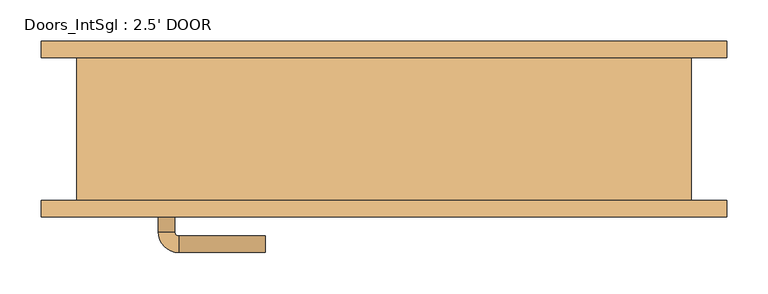
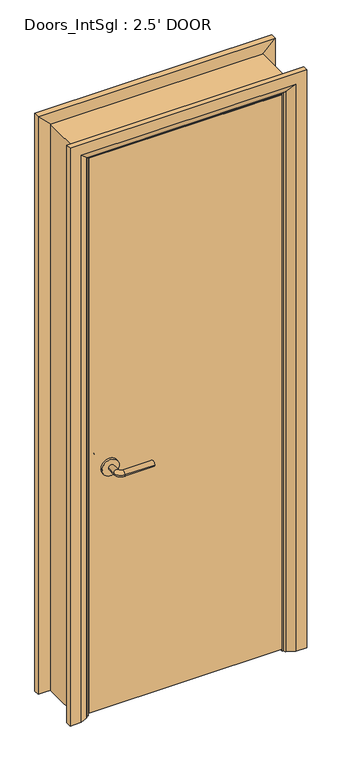
"""IFC4 building model written with IfcOpenShell, lengths in millimetres: door geometry, Doors_IntSgl : 2.5' DOOR."""

from ifc_helpers import new_model, si_unit, point, frame, frame_2d, origin, place, context, project, spatial, polyline, circle_curve, ellipse_curve, trimmed, segment, composite_curve, outline, extrude, faceted_brep, source, transform, mapped, element, save
from ifc_brep_helpers import plane_surface, cylinder_surface, revolved_surface, advanced_brep


def doors_intsgl_2_5_door_fd097d29(model_context):
    return source(origin(), model_context, "Body", "SolidModel", [
        advanced_brep(
        [(-274.0, -40.868, 900.0), (-254.0, -40.868, 900.0), (-274.0, -10.868, 900.0), (-254.0, -10.868, 900.0), (-249.0, -5.868, 900.0), (-249.0, 14.132, 900.0), (-144.0, 14.132, 900.0), (-144.0, -5.868, 900.0)],
        [
            (0, 1, circle_curve(frame((-264.0, -40.868, 900.0), z_axis=(0.0, -1.0, 0.0), x_axis=(1.0, 0.0, 0.0)), 10.0)),
            (1, 0, circle_curve(frame((-264.0, -40.868, 900.0), z_axis=(0.0, -1.0, 0.0), x_axis=(1.0, 0.0, 0.0)), 10.0)),
            (0, 2),
            (2, 3, circle_curve(frame((-264.0, -10.868, 900.0), z_axis=(0.0, -1.0, 0.0), x_axis=(1.0, 0.0, 0.0)), 10.0)),
            (3, 1),
            (3, 2, circle_curve(frame((-264.0, -10.868, 900.0), z_axis=(0.0, -1.0, 0.0), x_axis=(1.0, 0.0, 0.0)), 10.0)),
            (4, 3, circle_curve(frame((-249.0, -10.868, 900.0), z_axis=(0.0, 0.0, 1.0), x_axis=(-1.0, 0.0, 0.0)), 5.0)),
            (2, 5, circle_curve(frame((-249.0, -10.868, 900.0), z_axis=(0.0, 0.0, -1.0), x_axis=(-1.0, 0.0, 0.0)), 25.0)),
            (5, 4, circle_curve(frame((-249.0, 4.132, 900.0), z_axis=(-1.0, 0.0, 0.0), x_axis=(0.0, -1.0, 0.0)), 10.0)),
            (4, 5, circle_curve(frame((-249.0, 4.132, 900.0), z_axis=(-1.0, 0.0, 0.0), x_axis=(0.0, -1.0, 0.0)), 10.0)),
            (6, 7, circle_curve(frame((-144.0, 4.132, 900.0), z_axis=(1.0, 0.0, 0.0), x_axis=(0.0, -1.0, 0.0)), 10.0)),
            (7, 6, circle_curve(frame((-144.0, 4.132, 900.0), z_axis=(1.0, 0.0, 0.0), x_axis=(0.0, -1.0, 0.0)), 10.0)),
            (5, 6),
            (7, 4),
        ],
        [
            plane_surface(frame((-264.0, -40.868, 900.0), z_axis=(0.0, -1.0, 0.0), x_axis=(0.0, 0.0, 1.0))),
            cylinder_surface(frame((-264.0, -40.868, 900.0), z_axis=(0.0, -1.0, 0.0), x_axis=(1.0, 0.0, 0.0)), 10.0),
            revolved_surface(trimmed(ellipse_curve(frame((-264.0, -10.868, 900.0), z_axis=(0.0, -1.0, 0.0), x_axis=(1.0, 0.0, 0.0)), 10.0, 10.0), [point((-274.0, -10.868, 900.0))], [point((-254.0, -10.868, 900.0))], True, "CARTESIAN"), (-249.0, -10.868, 900.0), (0.0, 0.0, -1.0)),
            revolved_surface(trimmed(ellipse_curve(frame((-264.0, -10.868, 900.0), z_axis=(0.0, -1.0, 0.0), x_axis=(1.0, 0.0, 0.0)), 10.0, 10.0), [point((-254.0, -10.868, 900.0))], [point((-274.0, -10.868, 900.0))], True, "CARTESIAN"), (-249.0, -10.868, 900.0), (0.0, 0.0, -1.0)),
            plane_surface(frame((-144.0, 4.132, 900.0), z_axis=(1.0, 0.0, 0.0), x_axis=(0.0, 0.0, 1.0))),
            cylinder_surface(frame((-249.0, 4.132, 900.0), z_axis=(-1.0, 0.0, 0.0), x_axis=(0.0, -1.0, 0.0)), 10.0),
        ],
        [
            (0, [[1, 2]]),
            (1, [[-1, 3, 4, 5]]),
            (1, [[-2, -5, 6, -3]]),
            (2, [[7, -4, 8, 9]]),
            (3, [[-8, -6, -7, 10]]),
            (4, [[11, 12]]),
            (5, [[-9, 13, -12, 14]]),
            (5, [[-10, -14, -11, -13]]),
        ],
    ),
        extrude(outline(composite_curve([segment(trimmed(circle_curve(frame_2d((900.0, -266.5)), 30.0), [point((900.0, -296.5))], [point((900.0, -236.5))], False, "CARTESIAN"), True, "CONTINUOUS"), segment(trimmed(circle_curve(frame_2d((900.0, -266.5)), 30.0), [point((900.0, -236.5))], [point((900.0, -296.5))], False, "CARTESIAN"), True, "CONTINUOUS")], self_intersect=False)), frame((0.0, -48.868, 0.0), z_axis=(0.0, 1.0, 0.0), x_axis=(0.0, 0.0, 1.0)), (0.0, 0.0, 1.0), 8.0),
        advanced_brep(
        [(-274.0, -94.868, 900.0), (-254.0, -94.868, 900.0), (-254.0, -124.868, 900.0), (-274.0, -124.868, 900.0), (-249.0, -129.868, 900.0), (-249.0, -149.868, 900.0), (-144.0, -149.868, 900.0), (-144.0, -129.868, 900.0)],
        [
            (0, 1, circle_curve(frame((-264.0, -94.868, 900.0), z_axis=(0.0, 1.0, 0.0), x_axis=(1.0, 0.0, 0.0)), 10.0)),
            (1, 0, circle_curve(frame((-264.0, -94.868, 900.0), z_axis=(0.0, 1.0, 0.0), x_axis=(1.0, 0.0, 0.0)), 10.0)),
            (1, 2),
            (2, 3, circle_curve(frame((-264.0, -124.868, 900.0), z_axis=(0.0, 1.0, 0.0), x_axis=(1.0, 0.0, 0.0)), 10.0)),
            (3, 0),
            (3, 2, circle_curve(frame((-264.0, -124.868, 900.0), z_axis=(0.0, 1.0, 0.0), x_axis=(1.0, 0.0, 0.0)), 10.0)),
            (4, 5, circle_curve(frame((-249.0, -139.868, 900.0), z_axis=(-1.0, 0.0, 0.0), x_axis=(0.0, 1.0, 0.0)), 10.0)),
            (5, 3, circle_curve(frame((-249.0, -124.868, 900.0), z_axis=(0.0, 0.0, -1.0), x_axis=(-1.0, 0.0, 0.0)), 25.0)),
            (2, 4, circle_curve(frame((-249.0, -124.868, 900.0), z_axis=(0.0, 0.0, 1.0), x_axis=(-1.0, 0.0, 0.0)), 5.0)),
            (5, 4, circle_curve(frame((-249.0, -139.868, 900.0), z_axis=(-1.0, 0.0, 0.0), x_axis=(0.0, 1.0, 0.0)), 10.0)),
            (6, 7, circle_curve(frame((-144.0, -139.868, 900.0), z_axis=(1.0, 0.0, 0.0), x_axis=(0.0, 1.0, 0.0)), 10.0)),
            (7, 6, circle_curve(frame((-144.0, -139.868, 900.0), z_axis=(1.0, 0.0, 0.0), x_axis=(0.0, 1.0, 0.0)), 10.0)),
            (4, 7),
            (6, 5),
        ],
        [
            plane_surface(frame((-264.0, -94.868, 900.0), z_axis=(0.0, 1.0, 0.0), x_axis=(0.0, 0.0, 1.0))),
            cylinder_surface(frame((-264.0, -94.868, 900.0), z_axis=(0.0, 1.0, 0.0), x_axis=(1.0, 0.0, 0.0)), 10.0),
            revolved_surface(trimmed(ellipse_curve(frame((-264.0, -124.868, 900.0), z_axis=(0.0, -1.0, 0.0), x_axis=(1.0, 0.0, 0.0)), 10.0, 10.0), [point((-274.0, -124.868, 900.0))], [point((-254.0, -124.868, 900.0))], True, "CARTESIAN"), (-249.0, -124.868, 900.0), (0.0, 0.0, -1.0)),
            revolved_surface(trimmed(ellipse_curve(frame((-264.0, -124.868, 900.0), z_axis=(0.0, -1.0, 0.0), x_axis=(1.0, 0.0, 0.0)), 10.0, 10.0), [point((-254.0, -124.868, 900.0))], [point((-274.0, -124.868, 900.0))], True, "CARTESIAN"), (-249.0, -124.868, 900.0), (0.0, 0.0, -1.0)),
            plane_surface(frame((-144.0, -139.868, 900.0), z_axis=(1.0, 0.0, 0.0), x_axis=(0.0, 0.0, 1.0))),
            cylinder_surface(frame((-249.0, -139.868, 900.0), z_axis=(-1.0, 0.0, 0.0), x_axis=(0.0, 1.0, 0.0)), 10.0),
        ],
        [
            (0, [[1, 2]]),
            (1, [[3, 4, 5, -2]]),
            (1, [[-5, 6, -3, -1]]),
            (2, [[7, 8, -4, 9]]),
            (3, [[10, -9, -6, -8]]),
            (4, [[11, 12]]),
            (5, [[13, -11, 14, -7]]),
            (5, [[-14, -12, -13, -10]]),
        ],
    ),
        extrude(outline(composite_curve([segment(trimmed(circle_curve(frame_2d((900.0, -266.5)), 30.0), [point((900.0, -296.5))], [point((900.0, -236.5))], False, "CARTESIAN"), True, "CONTINUOUS"), segment(trimmed(circle_curve(frame_2d((900.0, -266.5)), 30.0), [point((900.0, -236.5))], [point((900.0, -296.5))], False, "CARTESIAN"), True, "CONTINUOUS")], self_intersect=False)), frame((0.0, -94.868, 0.0), z_axis=(0.0, 1.0, 0.0), x_axis=(0.0, 0.0, 1.0)), (0.0, 0.0, 1.0), 8.0),
        extrude(outline(polyline([(339.0, -48.868), (339.0, -86.868), (-339.0, -86.868), (-339.0, -48.868), (339.0, -48.868)])), frame((0.0, 0.0, 8.0), z_axis=(0.0, 0.0, 1.0), x_axis=(1.0, 0.0, 0.0)), (0.0, 0.0, 1.0), 2060.0),
        advanced_brep(
        [(416.0, -106.868, 0.0), (376.0, -106.868, 0.0), (350.0, -92.868, 0.0), (346.0, -86.868, 0.0), (416.0, -86.868, 0.0), (416.0, -86.868, 2145.0), (416.0, -106.868, 2145.0), (346.0, -86.868, 2075.0), (-346.0, -86.868, 2075.0), (-346.0, -86.868, 0.0), (-416.0, -86.868, 0.0), (-416.0, -86.868, 2145.0), (350.0, -92.868, 2079.0), (376.0, -106.868, 2105.0), (-416.0, -106.868, 2145.0), (-416.0, -106.868, 0.0), (-376.0, -106.868, 0.0), (-376.0, -106.868, 2105.0), (-350.0, -92.868, 0.0), (-350.0, -92.868, 2079.0)],
        [
            (0, 1),
            (1, 2),
            (2, 3, circle_curve(frame((354.0, -85.868, 0.0), z_axis=(0.0, 0.0, -1.0), x_axis=(1.0, 0.0, 0.0)), 8.0622577)),
            (3, 4),
            (4, 0),
            (4, 5),
            (5, 6),
            (6, 0),
            (3, 7),
            (7, 8),
            (8, 9),
            (9, 10),
            (10, 11),
            (11, 5),
            (2, 12),
            (12, 7, ellipse_curve(frame((354.0, -85.868, 2083.0), z_axis=(0.7071067811865475, 0.0, -0.7071067811865475), x_axis=(-0.7071067811865474, 0.0, -0.7071067811865476)), 11.4017543, 8.0622577)),
            (1, 13),
            (13, 12),
            (6, 14),
            (14, 15),
            (15, 16),
            (16, 17),
            (17, 13),
            (10, 15),
            (14, 11),
            (9, 18, circle_curve(frame((-354.0, -85.868, 0.0), z_axis=(0.0, 0.0, -1.0), x_axis=(-1.0, 0.0, 0.0)), 8.0622577)),
            (18, 16),
            (19, 18),
            (8, 19, ellipse_curve(frame((-354.0, -85.868, 2083.0), z_axis=(-0.7071067811865475, 0.0, -0.7071067811865475), x_axis=(-0.7071067811865474, 0.0, 0.7071067811865476)), 11.4017543, 8.0622577)),
            (19, 17),
            (12, 19),
        ],
        [
            plane_surface(frame((346.0, -86.868, 0.0), z_axis=(0.0, 0.0, -1.0), x_axis=(0.0, 1.0, 0.0))),
            plane_surface(frame((416.0, -106.868, 0.0), z_axis=(1.0, 0.0, 0.0), x_axis=(0.0, 0.0, 1.0))),
            plane_surface(frame((416.0, -86.868, 0.0), z_axis=(0.0, 1.0, 0.0), x_axis=(0.0, 0.0, 1.0))),
            cylinder_surface(frame((354.0, -85.868, 0.0), z_axis=(0.0, 0.0, -1.0), x_axis=(1.0, 0.0, 0.0)), 8.0622577),
            plane_surface(frame((350.0, -92.868, 0.0), z_axis=(-0.4740998230350126, -0.880471099922178, 0.0), x_axis=(0.0, 0.0, 1.0))),
            plane_surface(frame((376.0, -106.868, 0.0), z_axis=(0.0, -1.0, 0.0), x_axis=(0.0, 0.0, 1.0))),
            plane_surface(frame((-416.0, -106.868, 2145.0), z_axis=(-1.0, 0.0, 0.0), x_axis=(0.0, 0.0, -1.0))),
            plane_surface(frame((-346.0, -86.868, 0.0), z_axis=(0.0, 0.0, -1.0), x_axis=(0.0, 1.0, 0.0))),
            cylinder_surface(frame((-354.0, -85.868, 2075.0), z_axis=(0.0, 0.0, 1.0), x_axis=(-1.0, 0.0, 0.0)), 8.0622577),
            plane_surface(frame((-350.0, -92.868, 2079.0), z_axis=(0.47409982303501824, -0.8804710999221749, 0.0), x_axis=(0.0, 0.0, -1.0))),
            plane_surface(frame((416.0, -106.868, 2145.0), z_axis=(0.0, 0.0, 1.0), x_axis=(-1.0, 0.0, 0.0))),
            cylinder_surface(frame((346.0, -85.868, 2083.0), z_axis=(1.0, 0.0, 0.0), x_axis=(0.0, 0.0, 1.0)), 8.0622577),
            plane_surface(frame((350.0, -92.868, 2079.0), z_axis=(0.0, -0.8804710999221764, -0.4740998230350154), x_axis=(-1.0, 0.0, 0.0))),
        ],
        [
            (0, [[1, 2, 3, 4, 5]]),
            (1, [[6, 7, 8, -5]]),
            (2, [[9, 10, 11, 12, 13, 14, -6, -4]]),
            (3, [[15, 16, -9, -3]]),
            (4, [[17, 18, -15, -2]]),
            (5, [[-8, 19, 20, 21, 22, 23, -17, -1]]),
            (6, [[-13, 24, -20, 25]]),
            (7, [[-24, -12, 26, 27, -21]]),
            (8, [[28, -26, -11, 29]]),
            (9, [[-22, -27, -28, 30]]),
            (10, [[-14, -25, -19, -7]]),
            (11, [[31, -29, -10, -16]]),
            (12, [[-23, -30, -31, -18]]),
        ],
    ),
        extrude(outline(polyline([(0.0, -322.0), (2051.0, -322.0), (2051.0, 322.0), (0.0, 322.0), (0.0, 341.0), (2070.0, 341.0), (2070.0, -341.0), (0.0, -341.0), (0.0, -322.0)])), frame((0.0, -46.868, 0.0), z_axis=(0.0, 1.0, 0.0), x_axis=(0.0, 0.0, 1.0)), (0.0, 0.0, 1.0), 32.0),
        advanced_brep(
        [(-416.0, 106.868, 0.0), (-376.0, 106.868, 0.0), (-350.0, 92.868, 0.0), (-346.0, 86.868, 0.0), (-416.0, 86.868, 0.0), (-416.0, 86.868, 2145.0), (-416.0, 106.868, 2145.0), (-346.0, 86.868, 2075.0), (-350.0, 92.868, 2079.0), (-376.0, 106.868, 2105.0), (416.0, 106.868, 0.0), (416.0, 86.868, 0.0), (346.0, 86.868, 0.0), (350.0, 92.868, 0.0), (376.0, 106.868, 0.0), (416.0, 106.868, 2145.0), (376.0, 106.868, 2105.0), (350.0, 92.868, 2079.0), (346.0, 86.868, 2075.0), (416.0, 86.868, 2145.0)],
        [
            (0, 1),
            (1, 2),
            (2, 3, circle_curve(frame((-354.0, 85.868, 0.0), z_axis=(0.0, 0.0, -1.0), x_axis=(-1.0, 0.0, 0.0)), 8.0622577)),
            (3, 4),
            (4, 0),
            (4, 5),
            (5, 6),
            (6, 0),
            (3, 7),
            (7, 5),
            (2, 8),
            (8, 7, ellipse_curve(frame((-354.0, 85.868, 2083.0), z_axis=(-0.7071067811865475, 0.0, -0.7071067811865475), x_axis=(0.7071067811865474, 0.0, -0.7071067811865476)), 11.4017543, 8.0622577)),
            (1, 9),
            (9, 8),
            (6, 9),
            (10, 11),
            (11, 12),
            (12, 13, circle_curve(frame((354.0, 85.868, 0.0), z_axis=(0.0, 0.0, -1.0), x_axis=(1.0, 0.0, 0.0)), 8.0622577)),
            (13, 14),
            (14, 10),
            (15, 10),
            (14, 16),
            (16, 15),
            (13, 17),
            (17, 16),
            (12, 18),
            (18, 17, ellipse_curve(frame((354.0, 85.868, 2083.0), z_axis=(0.7071067811865475, 0.0, -0.7071067811865475), x_axis=(0.7071067811865474, 0.0, 0.7071067811865476)), 11.4017543, 8.0622577)),
            (11, 19),
            (19, 18),
            (15, 19),
            (5, 19),
            (15, 6),
            (7, 18),
            (8, 17),
            (9, 16),
        ],
        [
            plane_surface(frame((-346.0, 159.6690989, 0.0), z_axis=(0.0, 0.0, -1.0), x_axis=(1.0, 0.0, 0.0))),
            plane_surface(frame((-416.0, 106.868, 0.0), z_axis=(-1.0, 0.0, 0.0), x_axis=(0.0, 0.0, 1.0))),
            plane_surface(frame((-416.0, 86.868, 0.0), z_axis=(0.0, -1.0, 0.0), x_axis=(0.0, 0.0, 1.0))),
            cylinder_surface(frame((-354.0, 85.868, 0.0), z_axis=(0.0, 0.0, -1.0), x_axis=(-1.0, 0.0, 0.0)), 8.0622577),
            plane_surface(frame((-350.0, 92.868, 0.0), z_axis=(0.4740998230350183, 0.8804710999221749, 0.0), x_axis=(0.0, 0.0, 1.0))),
            plane_surface(frame((-376.0, 106.868, 0.0), z_axis=(0.0, 1.0, 0.0), x_axis=(0.0, 0.0, 1.0))),
            plane_surface(frame((346.0, 159.6690989, 0.0), z_axis=(0.0, 0.0, -1.0), x_axis=(-1.0, 0.0, 0.0))),
            plane_surface(frame((376.0, 106.868, 2105.0), z_axis=(0.0, 1.0, 0.0), x_axis=(0.0, 0.0, -1.0))),
            plane_surface(frame((350.0, 92.868, 2079.0), z_axis=(-0.4740998230350183, 0.8804710999221749, 0.0), x_axis=(0.0, 0.0, -1.0))),
            cylinder_surface(frame((354.0, 85.868, 2075.0), z_axis=(0.0, 0.0, 1.0), x_axis=(1.0, 0.0, 0.0)), 8.0622577),
            plane_surface(frame((416.0, 86.868, 2145.0), z_axis=(0.0, -1.0, 0.0), x_axis=(0.0, 0.0, -1.0))),
            plane_surface(frame((416.0, 106.868, 2145.0), z_axis=(1.0, 0.0, 0.0), x_axis=(0.0, 0.0, -1.0))),
            plane_surface(frame((-416.0, 106.868, 2145.0), z_axis=(0.0, 0.0, 1.0), x_axis=(1.0, 0.0, 0.0))),
            plane_surface(frame((-416.0, 86.868, 2145.0), z_axis=(0.0, -1.0, 0.0), x_axis=(1.0, 0.0, 0.0))),
            cylinder_surface(frame((-346.0, 85.868, 2083.0), z_axis=(-1.0, 0.0, 0.0), x_axis=(0.0, 0.0, 1.0)), 8.0622577),
            plane_surface(frame((-350.0, 92.868, 2079.0), z_axis=(0.0, 0.8804710999221749, -0.4740998230350183), x_axis=(1.0, 0.0, 0.0))),
            plane_surface(frame((-376.0, 106.868, 2105.0), z_axis=(0.0, 1.0, 0.0), x_axis=(1.0, 0.0, 0.0))),
        ],
        [
            (0, [[1, 2, 3, 4, 5]]),
            (1, [[6, 7, 8, -5]]),
            (2, [[9, 10, -6, -4]]),
            (3, [[11, 12, -9, -3]]),
            (4, [[13, 14, -11, -2]]),
            (5, [[-8, 15, -13, -1]]),
            (6, [[16, 17, 18, 19, 20]]),
            (7, [[21, -20, 22, 23]]),
            (8, [[-22, -19, 24, 25]]),
            (9, [[-24, -18, 26, 27]]),
            (10, [[-26, -17, 28, 29]]),
            (11, [[-28, -16, -21, 30]]),
            (12, [[31, -30, 32, -7]]),
            (13, [[33, -29, -31, -10]]),
            (14, [[34, -27, -33, -12]]),
            (15, [[35, -25, -34, -14]]),
            (16, [[-32, -23, -35, -15]]),
        ],
    ),
        faceted_brep([(-341.0, -86.868, 0.0), (-373.0, -86.868, 0.0), (-373.0, 86.868, 0.0), (-341.0, 86.868, 0.0), (-341.0, 86.868, 2070.0), (-341.0, -86.868, 2070.0), (-373.0, 86.868, 2102.0), (-373.0, -86.868, 2102.0), (341.0, -86.868, 0.0), (341.0, 86.868, 0.0), (373.0, 86.868, 0.0), (373.0, -86.868, 0.0), (341.0, -86.868, 2070.0), (373.0, -86.868, 2102.0), (373.0, 86.868, 2102.0), (341.0, 86.868, 2070.0)], [[[0, 1, 2, 3]], [[3, 4, 5, 0]], [[2, 6, 4, 3]], [[1, 7, 6, 2]], [[0, 5, 7, 1]], [[8, 9, 10, 11]], [[12, 8, 11, 13]], [[13, 11, 10, 14]], [[14, 10, 9, 15]], [[15, 9, 8, 12]], [[4, 15, 12, 5]], [[6, 14, 15, 4]], [[7, 13, 14, 6]], [[5, 12, 13, 7]]]),
    ])


if __name__ == "__main__":
    model = new_model("IFC4")
    model_context = context("Model", 3, world=origin())
    ifc_project = project(units=[si_unit("LENGTHUNIT", "METRE", prefix="MILLI")], contexts=[model_context])
    site = spatial("IfcSite", under=ifc_project)
    building = spatial("IfcBuilding", under=site)
    placement = place(None, origin())
    doors_intsgl_2_5_door_shape = doors_intsgl_2_5_door_fd097d29(model_context)
    element("IfcDoor", 1, ObjectType="Doors_IntSgl : 2.5' DOOR", at=placement, inside=building, context=model_context, shape_type="MappedRepresentation", body=[
        mapped(doors_intsgl_2_5_door_shape, transform((0.0, 0.0, 0.0), x_axis=(1.0, 0.0, 0.0), y_axis=(0.0, 1.0, 0.0), z_axis=(0.0, 0.0, 1.0))),
    ])
    save(model, "model.ifc")

# Revit data of these elements
# Type "Doors_IntSgl : 2.5' DOOR"
#   Type Mark = "47"
#   Type Comments = "Internal Single"
#   Operation = "SingleSwingRight"
#   Manufacturer = "Revit"
#   Keynote = "L20"
#   Description = "Internal Single Door"
#   Analytic Construction = "Metal"
#   UnderCut = 0.026247 ft
#   Tolerance = 0.006562 ft
#   Thickness = 0.124672 ft
#   Thermal Resistance (R) = 0.270117 (m²·K)/W
#   Structural Tolerance = 0.026247 ft
#   StopDepth = 0.104987 ft
#   Stop Thickness = 0.062336 ft
#   Rough Width = 2.5 ft
#   Rough Height = 6.922572 ft
#   Height to Top Lock Rail = 3.28084 ft
#   Heat Transfer Coefficient (U) = 3.7021 W/(m²·K)
#   Handle Z Distance = 2.952756 ft
#   Handle X Distance = 0.246063 ft
#   Frame Thickness = 0.104987 ft
#   Door Panel Width = 2.224409 ft
#   Door Panel Thickness = 0.124672 ft
#   Door Panel Offset = 0.0 ft
#   Height = 6.922572 ft
#   Width = 2.5 ft
#   Door Panel Height = 6.75853 ft
#   Architrave Setback = 0.016404 ft
#   Vis - Ironmongery = yes
#   Material Ironmongery = Door - Handle
#   Material Frame = Door - Frame/Mullion (1)
#   Material Door = Door - Panel
#   Material Architrave = Door - Architrave
#   Visual Light Transmittance = 0
#   Solar Heat Gain Coefficient = 0
#   Function = (empty or 0)
#   Wall Closure = (empty or 0)
# Element 1 (IfcDoor, "Doors_IntSgl : 2.5' DOOR")
#   Materials on its faces: "Door - Architrave", "Door - Handle", "Door - Frame/Mullion (1)", "Door - Panel"
# Materials
#   "Door - Handle": colour RGB 0 0 0, transparency 0, Keynote = "P21", Cost = 0
#   "Door - Frame/Mullion (1)": class "Wood", colour RGB 212 179 113, transparency 0, Keynote = "L20", Cost = 0
#   "Door - Panel": class "Wood", colour RGB 210 159 95, transparency 0, Keynote = "L20", Cost = 0
#   "Door - Architrave": class "Wood", colour RGB 154 90 5, transparency 0, Keynote = "P20", Cost = 0
